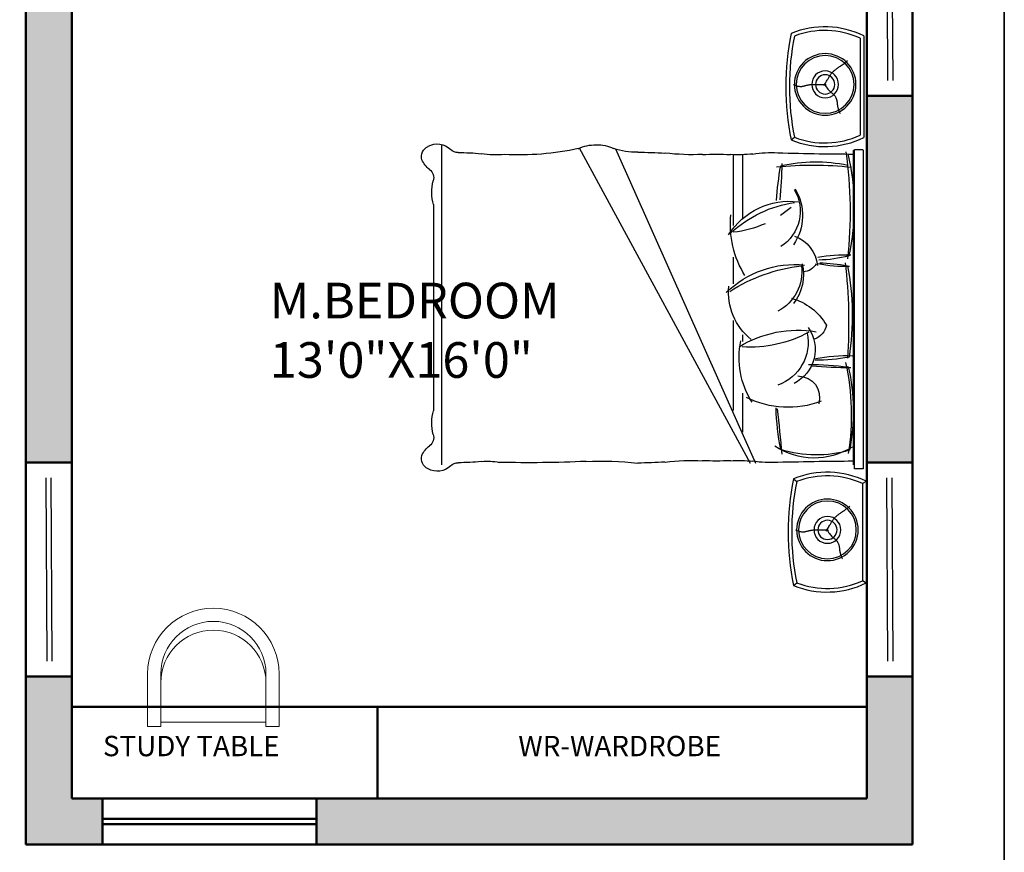
# Model space of a CAD drawing. Units: inches. Extents: x 1986 to 21484, y -1816 to 2016.
# Tile 3 of 85: x 2209 to 2402, y 1113 to 1277. Entities that reach past the tile are written whole.
import ezdxf

# ---------------------------------------------------------------- set-up
doc = ezdxf.new("R2010")
doc.units = ezdxf.units.IN
for name, color, linetype, lineweight in [('A-ANNO-TEXT', 7, 'Continuous', 18), ('A-AREA-IDEN', 3, 'Continuous', 18), ('A-FLOR-FIXT', 8, 'Continuous', 18), ('A-FURN', 8, 'Continuous', 18), ('A-GLAZ', 4, 'Continuous', 25), ('A-WALL', 7, 'Continuous', 50), ('A-WALL-PATT', 8, 'Continuous', 13), ('C-PROP', 7, 'Continuous', 35)]:
    doc.layers.add(name, color=color, linetype=linetype, lineweight=lineweight)
doc.layers.add('TEFRİŞ', color=11, linetype='Continuous')
doc.styles.get("Standard").update_dxf_attribs({"font": 'arial.ttf'})

# ---------------------------------------------------------------- blocks, each defined once
blk = doc.blocks.new('12PSTG07')
at = {"color": 0, "linetype": 'ByBlock'}
for p, q in [((0, 15), (-12, 15)), ((0, 12), (0, 15)), ((-12, 12), (0, 12)), ((-1, -12), (-1, 12)), ((-12, -12), (0, -12)), ((0, -12), (0, -15)), ((0, -15), (-12, -15))]:
    blk.add_line(p, q, dxfattribs=at)
for centre, radius in [((-12, 0), 15), ((-12, 0), 12), ((-10, 0), 12)]:
    blk.add_arc(centre, radius, 90, 270, dxfattribs=at)
blk = doc.blocks.new('BED')
at = {"layer": 'TEFRİŞ'}
for p, q in [((2114.88, 1835.66), (2129.12, 1835.66)), ((2130.81, 1834.34), (2130.81, 1835.55)), ((2130.91, 1835.55), (2175.56, 1835.55)), ((2175.56, 1835.55), (2175.56, 1834.34)), ((2177.29, 1835.98), (2177.61, 1835.47)), ((2177.29, 1835.98), (2191.52, 1835.98)), ((2177.61, 1835.47), (2191.2, 1835.47)), ((2191.2, 1835.47), (2191.52, 1835.98)), ((2115.2, 1835.15), (2128.8, 1835.15)), ((2175.56, 1834.34), (2130.81, 1834.34)), ((2175, 1834.19), (2130.91, 1834.19)), ((2118.49, 1833.2), (2118.34, 1833.38)), ((2118.49, 1833.2), (2118.34, 1833.38)), ((2118.63, 1833.03), (2118.49, 1833.2)), ((2118.63, 1833.03), (2118.49, 1833.2)), ((2118.75, 1832.88), (2118.63, 1833.03)), ((2118.75, 1832.88), (2118.63, 1833.03)), ((2118.86, 1832.74), (2118.75, 1832.88)), ((2118.86, 1832.74), (2118.75, 1832.88)), ((2118.95, 1832.61), (2118.86, 1832.74)), ((2118.95, 1832.61), (2118.86, 1832.74)), ((2119.04, 1832.48), (2118.95, 1832.61)), ((2119.04, 1832.48), (2118.95, 1832.61)), ((2180.9, 1833.52), (2180.75, 1833.7)), ((2180.9, 1833.52), (2180.75, 1833.7)), ((2181.04, 1833.35), (2180.9, 1833.52)), ((2181.04, 1833.35), (2180.9, 1833.52)), ((2181.16, 1833.2), (2181.04, 1833.35)), ((2181.16, 1833.2), (2181.04, 1833.35)), ((2181.26, 1833.06), (2181.16, 1833.2)), ((2181.26, 1833.06), (2181.16, 1833.2)), ((2181.36, 1832.93), (2181.26, 1833.06)), ((2181.36, 1832.93), (2181.26, 1833.06)), ((2181.44, 1832.8), (2181.36, 1832.93)), ((2181.44, 1832.8), (2181.36, 1832.93)), ((2181.52, 1832.69), (2181.44, 1832.8)), ((2181.52, 1832.69), (2181.44, 1832.8)), ((2181.59, 1832.58), (2181.52, 1832.69)), ((2181.59, 1832.58), (2181.52, 1832.69)), ((2181.66, 1832.48), (2181.59, 1832.58)), ((2181.66, 1832.48), (2181.59, 1832.58)), ((2187.83, 1832.49), (2187.92, 1832.53)), ((2187.83, 1832.49), (2187.92, 1832.53)), ((2187.92, 1832.53), (2188.01, 1832.57)), ((2187.92, 1832.53), (2188.01, 1832.57)), ((2188.01, 1832.57), (2188.09, 1832.62)), ((2188.01, 1832.57), (2188.09, 1832.62)), ((2188.09, 1832.62), (2188.15, 1832.67)), ((2188.09, 1832.62), (2188.15, 1832.67)), ((2119.12, 1832.37), (2119.04, 1832.48)), ((2119.12, 1832.37), (2119.04, 1832.48)), ((2119.19, 1832.26), (2119.12, 1832.37)), ((2119.19, 1832.26), (2119.12, 1832.37)), ((2119.26, 1832.16), (2119.19, 1832.26)), ((2119.26, 1832.16), (2119.19, 1832.26)), ((2119.32, 1832.06), (2119.26, 1832.16)), ((2119.32, 1832.06), (2119.26, 1832.16)), ((2119.39, 1831.97), (2119.32, 1832.06)), ((2119.39, 1831.97), (2119.32, 1832.06)), ((2119.45, 1831.89), (2119.39, 1831.97)), ((2119.45, 1831.89), (2119.39, 1831.97)), ((2119.51, 1831.81), (2119.45, 1831.89)), ((2119.51, 1831.81), (2119.45, 1831.89)), ((2119.57, 1831.73), (2119.51, 1831.81)), ((2119.57, 1831.73), (2119.51, 1831.81)), ((2119.63, 1831.65), (2119.57, 1831.73)), ((2119.63, 1831.65), (2119.57, 1831.73)), ((2119.69, 1831.58), (2119.63, 1831.65)), ((2119.69, 1831.58), (2119.63, 1831.65)), ((2119.75, 1831.51), (2119.69, 1831.58)), ((2119.75, 1831.51), (2119.69, 1831.58)), ((2119.81, 1831.44), (2119.75, 1831.51)), ((2119.81, 1831.44), (2119.75, 1831.51)), ((2119.87, 1831.38), (2119.81, 1831.44)), ((2119.87, 1831.38), (2119.81, 1831.44)), ((2119.93, 1831.31), (2119.87, 1831.38)), ((2119.93, 1831.31), (2119.87, 1831.38)), ((2119.99, 1831.25), (2119.93, 1831.31)), ((2119.99, 1831.25), (2119.93, 1831.31)), ((2120.05, 1831.2), (2119.99, 1831.25)), ((2120.05, 1831.2), (2119.99, 1831.25)), ((2120.12, 1831.14), (2120.05, 1831.2)), ((2120.12, 1831.14), (2120.05, 1831.2)), ((2120.18, 1831.09), (2120.12, 1831.14)), ((2120.18, 1831.09), (2120.12, 1831.14)), ((2122.8, 1831.09), (2122.87, 1831.18)), ((2122.8, 1831.09), (2122.87, 1831.18)), ((2122.87, 1831.18), (2122.94, 1831.26)), ((2122.87, 1831.18), (2122.94, 1831.26)), ((2122.94, 1831.26), (2123.01, 1831.33)), ((2122.94, 1831.26), (2123.01, 1831.33)), ((2123.01, 1831.33), (2123.08, 1831.4)), ((2123.01, 1831.33), (2123.08, 1831.4)), ((2123.08, 1831.4), (2123.14, 1831.46)), ((2123.08, 1831.4), (2123.14, 1831.46)), ((2123.14, 1831.46), (2123.21, 1831.52)), ((2123.14, 1831.46), (2123.21, 1831.52)), ((2123.21, 1831.52), (2123.27, 1831.58)), ((2123.21, 1831.52), (2123.27, 1831.58)), ((2123.27, 1831.58), (2123.34, 1831.63)), ((2123.27, 1831.58), (2123.34, 1831.63)), ((2123.34, 1831.63), (2123.41, 1831.67)), ((2123.34, 1831.63), (2123.41, 1831.67)), ((2123.41, 1831.67), (2123.48, 1831.71)), ((2123.41, 1831.67), (2123.48, 1831.71)), ((2123.48, 1831.71), (2123.55, 1831.74)), ((2123.48, 1831.71), (2123.55, 1831.74)), ((2123.55, 1831.74), (2123.62, 1831.77)), ((2123.55, 1831.74), (2123.62, 1831.77)), ((2123.62, 1831.77), (2123.69, 1831.8)), ((2123.62, 1831.77), (2123.69, 1831.8)), ((2123.69, 1831.8), (2123.77, 1831.82)), ((2123.69, 1831.8), (2123.77, 1831.82)), ((2123.77, 1831.82), (2123.84, 1831.84)), ((2123.77, 1831.82), (2123.84, 1831.84)), ((2123.84, 1831.84), (2123.91, 1831.86)), ((2123.84, 1831.84), (2123.91, 1831.86)), ((2123.91, 1831.86), (2123.98, 1831.87)), ((2123.91, 1831.86), (2123.98, 1831.87)), ((2123.98, 1831.87), (2124.06, 1831.89)), ((2123.98, 1831.87), (2124.06, 1831.89)), ((2124.06, 1831.89), (2124.13, 1831.9)), ((2124.06, 1831.89), (2124.13, 1831.9)), ((2124.13, 1831.9), (2124.2, 1831.91)), ((2124.13, 1831.9), (2124.2, 1831.91)), ((2124.2, 1831.91), (2124.27, 1831.91)), ((2124.2, 1831.91), (2124.27, 1831.91)), ((2124.27, 1831.91), (2124.35, 1831.92)), ((2124.27, 1831.91), (2124.35, 1831.92)), ((2124.35, 1831.92), (2124.42, 1831.93)), ((2124.35, 1831.92), (2124.42, 1831.93)), ((2124.42, 1831.93), (2124.49, 1831.94)), ((2124.42, 1831.93), (2124.49, 1831.94)), ((2124.49, 1831.94), (2124.56, 1831.95)), ((2124.49, 1831.94), (2124.56, 1831.95)), ((2124.56, 1831.95), (2124.64, 1831.96)), ((2124.56, 1831.95), (2124.64, 1831.96)), ((2124.64, 1831.96), (2124.71, 1831.98)), ((2124.64, 1831.96), (2124.71, 1831.98)), ((2124.71, 1831.98), (2124.79, 1831.99)), ((2124.71, 1831.98), (2124.79, 1831.99)), ((2124.79, 1831.99), (2124.87, 1832.01)), ((2124.79, 1831.99), (2124.87, 1832.01)), ((2124.87, 1832.01), (2124.96, 1832.03)), ((2124.87, 1832.01), (2124.96, 1832.03)), ((2124.96, 1832.03), (2125.05, 1832.05)), ((2124.96, 1832.03), (2125.05, 1832.05)), ((2125.05, 1832.05), (2125.14, 1832.08)), ((2125.05, 1832.05), (2125.14, 1832.08)), ((2125.14, 1832.08), (2125.23, 1832.11)), ((2125.14, 1832.08), (2125.23, 1832.11)), ((2125.23, 1832.11), (2125.33, 1832.14)), ((2125.23, 1832.11), (2125.33, 1832.14)), ((2125.33, 1832.14), (2125.42, 1832.17)), ((2125.33, 1832.14), (2125.42, 1832.17)), ((2125.42, 1832.17), (2125.52, 1832.21)), ((2125.42, 1832.17), (2125.52, 1832.21)), ((2125.52, 1832.21), (2125.6, 1832.25)), ((2125.52, 1832.21), (2125.6, 1832.25)), ((2125.6, 1832.25), (2125.68, 1832.3)), ((2125.6, 1832.25), (2125.68, 1832.3)), ((2125.68, 1832.3), (2125.75, 1832.35)), ((2125.68, 1832.3), (2125.75, 1832.35)), ((2181.73, 1832.38), (2181.66, 1832.48)), ((2181.73, 1832.38), (2181.66, 1832.48)), ((2181.79, 1832.29), (2181.73, 1832.38)), ((2181.79, 1832.29), (2181.73, 1832.38)), ((2181.85, 1832.21), (2181.79, 1832.29)), ((2181.85, 1832.21), (2181.79, 1832.29)), ((2181.92, 1832.13), (2181.85, 1832.21)), ((2181.92, 1832.13), (2181.85, 1832.21)), ((2181.97, 1832.05), (2181.92, 1832.13)), ((2181.97, 1832.05), (2181.92, 1832.13)), ((2182.03, 1831.97), (2181.97, 1832.05)), ((2182.03, 1831.97), (2181.97, 1832.05)), ((2182.09, 1831.9), (2182.03, 1831.97)), ((2182.09, 1831.9), (2182.03, 1831.97)), ((2182.15, 1831.83), (2182.09, 1831.9)), ((2182.15, 1831.83), (2182.09, 1831.9)), ((2182.21, 1831.76), (2182.15, 1831.83)), ((2182.21, 1831.76), (2182.15, 1831.83)), ((2182.27, 1831.7), (2182.21, 1831.76)), ((2182.27, 1831.7), (2182.21, 1831.76)), ((2182.33, 1831.63), (2182.27, 1831.7)), ((2182.33, 1831.63), (2182.27, 1831.7)), ((2182.4, 1831.57), (2182.33, 1831.63)), ((2182.4, 1831.57), (2182.33, 1831.63)), ((2182.46, 1831.52), (2182.4, 1831.57)), ((2182.46, 1831.52), (2182.4, 1831.57)), ((2182.52, 1831.46), (2182.46, 1831.52)), ((2182.52, 1831.46), (2182.46, 1831.52)), ((2182.59, 1831.41), (2182.52, 1831.46)), ((2182.59, 1831.41), (2182.52, 1831.46)), ((2182.66, 1831.36), (2182.59, 1831.41)), ((2182.66, 1831.36), (2182.59, 1831.41)), ((2182.73, 1831.31), (2182.66, 1831.36)), ((2182.73, 1831.31), (2182.66, 1831.36)), ((2182.8, 1831.26), (2182.73, 1831.31)), ((2182.8, 1831.26), (2182.73, 1831.31)), ((2182.87, 1831.22), (2182.8, 1831.26)), ((2182.87, 1831.22), (2182.8, 1831.26)), ((2182.95, 1831.17), (2182.87, 1831.22)), ((2182.95, 1831.17), (2182.87, 1831.22)), ((2183.03, 1831.12), (2182.95, 1831.17)), ((2183.03, 1831.12), (2182.95, 1831.17)), ((2184.85, 1831.04), (2184.95, 1831.14)), ((2184.85, 1831.04), (2184.95, 1831.14)), ((2184.95, 1831.14), (2185.05, 1831.23)), ((2184.95, 1831.14), (2185.05, 1831.23)), ((2185.05, 1831.23), (2185.13, 1831.33)), ((2185.05, 1831.23), (2185.13, 1831.33)), ((2185.13, 1831.33), (2185.21, 1831.41)), ((2185.13, 1831.33), (2185.21, 1831.41)), ((2185.21, 1831.41), (2185.28, 1831.5)), ((2185.21, 1831.41), (2185.28, 1831.5)), ((2185.28, 1831.5), (2185.35, 1831.58)), ((2185.28, 1831.5), (2185.35, 1831.58)), ((2185.35, 1831.58), (2185.42, 1831.65)), ((2185.35, 1831.58), (2185.42, 1831.65)), ((2185.42, 1831.65), (2185.48, 1831.72)), ((2185.42, 1831.65), (2185.48, 1831.72)), ((2185.48, 1831.72), (2185.55, 1831.78)), ((2185.48, 1831.72), (2185.55, 1831.78)), ((2185.55, 1831.78), (2185.61, 1831.84)), ((2185.55, 1831.78), (2185.61, 1831.84)), ((2185.61, 1831.84), (2185.68, 1831.9)), ((2185.61, 1831.84), (2185.68, 1831.9)), ((2185.68, 1831.9), (2185.75, 1831.95)), ((2185.68, 1831.9), (2185.75, 1831.95)), ((2185.75, 1831.95), (2185.82, 1831.99)), ((2185.75, 1831.95), (2185.82, 1831.99)), ((2185.82, 1831.99), (2185.89, 1832.03)), ((2185.82, 1831.99), (2185.89, 1832.03)), ((2185.89, 1832.03), (2185.96, 1832.06)), ((2185.89, 1832.03), (2185.96, 1832.06)), ((2185.96, 1832.06), (2186.03, 1832.09)), ((2185.96, 1832.06), (2186.03, 1832.09)), ((2186.03, 1832.09), (2186.1, 1832.12)), ((2186.03, 1832.09), (2186.1, 1832.12)), ((2186.1, 1832.12), (2186.17, 1832.14)), ((2186.1, 1832.12), (2186.17, 1832.14)), ((2186.17, 1832.14), (2186.24, 1832.16)), ((2186.17, 1832.14), (2186.24, 1832.16)), ((2186.24, 1832.16), (2186.32, 1832.18)), ((2186.24, 1832.16), (2186.32, 1832.18)), ((2186.32, 1832.18), (2186.39, 1832.19)), ((2186.32, 1832.18), (2186.39, 1832.19)), ((2186.39, 1832.19), (2186.46, 1832.21)), ((2186.39, 1832.19), (2186.46, 1832.21)), ((2186.46, 1832.21), (2186.53, 1832.22)), ((2186.46, 1832.21), (2186.53, 1832.22)), ((2186.53, 1832.22), (2186.61, 1832.23)), ((2186.53, 1832.22), (2186.61, 1832.23)), ((2186.61, 1832.23), (2186.68, 1832.23)), ((2186.61, 1832.23), (2186.68, 1832.23)), ((2186.68, 1832.23), (2186.75, 1832.24)), ((2186.68, 1832.23), (2186.75, 1832.24)), ((2186.75, 1832.24), (2186.82, 1832.25)), ((2186.75, 1832.24), (2186.82, 1832.25)), ((2186.82, 1832.25), (2186.9, 1832.26)), ((2186.82, 1832.25), (2186.9, 1832.26)), ((2186.9, 1832.26), (2186.97, 1832.27)), ((2186.9, 1832.26), (2186.97, 1832.27)), ((2186.97, 1832.27), (2187.04, 1832.28)), ((2186.97, 1832.27), (2187.04, 1832.28)), ((2187.04, 1832.28), (2187.12, 1832.3)), ((2187.04, 1832.28), (2187.12, 1832.3)), ((2187.12, 1832.3), (2187.2, 1832.31)), ((2187.12, 1832.3), (2187.2, 1832.31)), ((2187.2, 1832.31), (2187.28, 1832.33)), ((2187.2, 1832.31), (2187.28, 1832.33)), ((2187.28, 1832.33), (2187.36, 1832.35)), ((2187.28, 1832.33), (2187.36, 1832.35)), ((2187.36, 1832.35), (2187.45, 1832.37)), ((2187.36, 1832.35), (2187.45, 1832.37)), ((2187.45, 1832.37), (2187.54, 1832.4)), ((2187.45, 1832.37), (2187.54, 1832.4)), ((2187.54, 1832.4), (2187.64, 1832.43)), ((2187.54, 1832.4), (2187.64, 1832.43)), ((2187.64, 1832.43), (2187.74, 1832.46)), ((2187.64, 1832.43), (2187.74, 1832.46)), ((2187.74, 1832.46), (2187.83, 1832.49)), ((2187.74, 1832.46), (2187.83, 1832.49)), ((2120.25, 1831.04), (2120.18, 1831.09)), ((2120.25, 1831.04), (2120.18, 1831.09)), ((2120.32, 1830.99), (2120.25, 1831.04)), ((2120.32, 1830.99), (2120.25, 1831.04)), ((2120.39, 1830.94), (2120.32, 1830.99)), ((2120.39, 1830.94), (2120.32, 1830.99)), ((2120.47, 1830.9), (2120.39, 1830.94)), ((2120.47, 1830.9), (2120.39, 1830.94)), ((2120.54, 1830.85), (2120.47, 1830.9)), ((2120.54, 1830.85), (2120.47, 1830.9)), ((2120.62, 1830.8), (2120.54, 1830.85)), ((2120.62, 1830.8), (2120.54, 1830.85)), ((2120.7, 1830.75), (2120.62, 1830.8)), ((2120.7, 1830.75), (2120.62, 1830.8)), ((2120.79, 1830.7), (2120.7, 1830.75)), ((2120.79, 1830.7), (2120.7, 1830.75)), ((2120.88, 1830.65), (2120.79, 1830.7)), ((2120.88, 1830.65), (2120.79, 1830.7)), ((2120.98, 1830.59), (2120.88, 1830.65)), ((2120.98, 1830.59), (2120.88, 1830.65)), ((2121.09, 1830.52), (2120.98, 1830.59)), ((2121.09, 1830.52), (2120.98, 1830.59)), ((2121.21, 1830.45), (2121.09, 1830.52)), ((2121.21, 1830.45), (2121.09, 1830.52)), ((2121.34, 1830.38), (2121.21, 1830.45)), ((2121.34, 1830.38), (2121.21, 1830.45)), ((2121.49, 1830.29), (2121.34, 1830.38)), ((2121.49, 1830.29), (2121.34, 1830.38)), ((2121.66, 1830.21), (2121.49, 1830.29)), ((2121.66, 1830.21), (2121.49, 1830.29)), ((2121.66, 1830.18), (2121.87, 1830.29)), ((2121.66, 1830.18), (2121.87, 1830.29)), ((2121.85, 1830.11), (2121.66, 1830.21)), ((2121.85, 1830.11), (2121.66, 1830.21)), ((2121.74, 1829.99), (2121.73, 1829.83)), ((2121.74, 1829.99), (2121.73, 1829.83)), ((2121.73, 1829.83), (2121.73, 1829.69)), ((2121.73, 1829.83), (2121.73, 1829.69)), ((2121.76, 1830.38), (2121.74, 1830.17)), ((2121.76, 1830.38), (2121.74, 1830.17)), ((2121.74, 1830.17), (2121.74, 1829.99)), ((2121.74, 1830.17), (2121.74, 1829.99)), ((2121.87, 1830.29), (2122.04, 1830.4)), ((2121.87, 1830.29), (2122.04, 1830.4)), ((2122.04, 1830.4), (2122.2, 1830.51)), ((2122.04, 1830.4), (2122.2, 1830.51)), ((2122.2, 1830.51), (2122.33, 1830.61)), ((2122.2, 1830.51), (2122.33, 1830.61)), ((2122.33, 1830.61), (2122.45, 1830.72)), ((2122.33, 1830.61), (2122.45, 1830.72)), ((2122.45, 1830.72), (2122.55, 1830.82)), ((2122.45, 1830.72), (2122.55, 1830.82)), ((2122.55, 1830.82), (2122.64, 1830.91)), ((2122.55, 1830.82), (2122.64, 1830.91)), ((2122.64, 1830.91), (2122.72, 1831.01)), ((2122.64, 1830.91), (2122.72, 1831.01)), ((2122.72, 1831.01), (2122.8, 1831.09)), ((2122.72, 1831.01), (2122.8, 1831.09)), ((2183.11, 1831.07), (2183.03, 1831.12)), ((2183.11, 1831.07), (2183.03, 1831.12)), ((2183.2, 1831.02), (2183.11, 1831.07)), ((2183.2, 1831.02), (2183.11, 1831.07)), ((2183.29, 1830.97), (2183.2, 1831.02)), ((2183.29, 1830.97), (2183.2, 1831.02)), ((2183.39, 1830.91), (2183.29, 1830.97)), ((2183.39, 1830.91), (2183.29, 1830.97)), ((2183.49, 1830.84), (2183.39, 1830.91)), ((2183.49, 1830.84), (2183.39, 1830.91)), ((2183.61, 1830.77), (2183.49, 1830.84)), ((2183.61, 1830.77), (2183.49, 1830.84)), ((2183.75, 1830.7), (2183.61, 1830.77)), ((2183.75, 1830.7), (2183.61, 1830.77)), ((2183.9, 1830.61), (2183.75, 1830.7)), ((2183.9, 1830.61), (2183.75, 1830.7)), ((2184.06, 1830.53), (2183.9, 1830.61)), ((2184.06, 1830.53), (2183.9, 1830.61)), ((2184.25, 1830.43), (2184.06, 1830.53)), ((2184.25, 1830.43), (2184.06, 1830.53)), ((2184.07, 1830.5), (2184.27, 1830.61)), ((2184.07, 1830.5), (2184.27, 1830.61)), ((2184.15, 1830.49), (2184.14, 1830.31)), ((2184.15, 1830.49), (2184.14, 1830.31)), ((2184.14, 1830.31), (2184.14, 1830.15)), ((2184.14, 1830.31), (2184.14, 1830.15)), ((2184.14, 1830.15), (2184.14, 1830.01)), ((2184.14, 1830.15), (2184.14, 1830.01)), ((2184.14, 1830.01), (2184.14, 1829.89)), ((2184.14, 1830.01), (2184.14, 1829.89)), ((2184.14, 1829.89), (2184.14, 1829.77)), ((2184.14, 1829.89), (2184.14, 1829.77)), ((2184.14, 1829.77), (2184.14, 1829.67)), ((2184.14, 1829.77), (2184.14, 1829.67)), ((2184.17, 1830.7), (2184.15, 1830.49)), ((2184.17, 1830.7), (2184.15, 1830.49)), ((2184.27, 1830.61), (2184.45, 1830.72)), ((2184.27, 1830.61), (2184.45, 1830.72)), ((2184.45, 1830.72), (2184.6, 1830.83)), ((2184.45, 1830.72), (2184.6, 1830.83)), ((2184.6, 1830.83), (2184.74, 1830.93)), ((2184.6, 1830.83), (2184.74, 1830.93)), ((2184.74, 1830.93), (2184.85, 1831.04)), ((2184.74, 1830.93), (2184.85, 1831.04)), ((2121.73, 1829.69), (2121.73, 1829.57)), ((2121.73, 1829.69), (2121.73, 1829.57)), ((2121.73, 1829.57), (2121.73, 1829.45)), ((2121.73, 1829.57), (2121.73, 1829.45)), ((2121.73, 1829.45), (2121.74, 1829.35)), ((2121.73, 1829.45), (2121.74, 1829.35)), ((2121.74, 1828.89), (2121.73, 1828.8)), ((2121.74, 1828.89), (2121.73, 1828.8)), ((2121.73, 1828.8), (2121.73, 1828.72)), ((2121.73, 1828.8), (2121.73, 1828.72)), ((2121.73, 1828.72), (2121.73, 1828.64)), ((2121.73, 1828.72), (2121.73, 1828.64)), ((2121.73, 1828.64), (2121.73, 1828.56)), ((2121.73, 1828.64), (2121.73, 1828.56)), ((2121.73, 1828.56), (2121.73, 1828.48)), ((2121.73, 1828.56), (2121.73, 1828.48)), ((2121.73, 1828.48), (2121.73, 1828.4)), ((2121.73, 1828.48), (2121.73, 1828.4)), ((2121.73, 1828.4), (2121.73, 1828.33)), ((2121.73, 1828.4), (2121.73, 1828.33)), ((2121.74, 1829.35), (2121.74, 1829.25)), ((2121.74, 1829.35), (2121.74, 1829.25)), ((2121.74, 1829.25), (2121.74, 1829.16)), ((2121.74, 1829.25), (2121.74, 1829.16)), ((2121.74, 1829.16), (2121.74, 1829.06)), ((2121.74, 1829.16), (2121.74, 1829.06)), ((2121.74, 1829.06), (2121.74, 1828.97)), ((2121.74, 1829.06), (2121.74, 1828.97)), ((2121.74, 1828.97), (2121.74, 1828.89)), ((2121.74, 1828.97), (2121.74, 1828.89)), ((2184.14, 1829.04), (2184.13, 1828.96)), ((2184.14, 1829.04), (2184.13, 1828.96)), ((2184.13, 1828.96), (2184.13, 1828.88)), ((2184.13, 1828.96), (2184.13, 1828.88)), ((2184.13, 1828.88), (2184.13, 1828.8)), ((2184.13, 1828.88), (2184.13, 1828.8)), ((2184.13, 1828.8), (2184.14, 1828.72)), ((2184.13, 1828.8), (2184.14, 1828.72)), ((2184.14, 1829.67), (2184.15, 1829.57)), ((2184.14, 1829.67), (2184.15, 1829.57)), ((2184.15, 1829.38), (2184.14, 1829.29)), ((2184.15, 1829.38), (2184.14, 1829.29)), ((2184.14, 1829.29), (2184.14, 1829.21)), ((2184.14, 1829.29), (2184.14, 1829.21)), ((2184.14, 1829.21), (2184.14, 1829.12)), ((2184.14, 1829.21), (2184.14, 1829.12)), ((2184.14, 1829.12), (2184.14, 1829.04)), ((2184.14, 1829.12), (2184.14, 1829.04)), ((2184.14, 1828.72), (2184.14, 1828.65)), ((2184.14, 1828.72), (2184.14, 1828.65)), ((2184.14, 1828.65), (2184.15, 1828.57)), ((2184.14, 1828.65), (2184.15, 1828.57)), ((2184.15, 1829.57), (2184.15, 1829.48)), ((2184.15, 1829.57), (2184.15, 1829.48)), ((2184.15, 1829.48), (2184.15, 1829.38)), ((2184.15, 1829.48), (2184.15, 1829.38)), ((2184.15, 1828.57), (2184.15, 1828.5)), ((2184.15, 1828.57), (2184.15, 1828.5)), ((2184.15, 1828.5), (2184.16, 1828.42)), ((2184.15, 1828.5), (2184.16, 1828.42)), ((2184.16, 1828.42), (2184.17, 1828.35)), ((2184.16, 1828.42), (2184.17, 1828.35)), ((2121.73, 1828.33), (2121.74, 1828.25)), ((2121.73, 1828.33), (2121.74, 1828.25)), ((2121.74, 1828.25), (2121.75, 1828.18)), ((2121.74, 1828.25), (2121.75, 1828.18)), ((2121.75, 1828.18), (2121.75, 1828.1)), ((2121.75, 1828.18), (2121.75, 1828.1)), ((2121.75, 1828.1), (2121.76, 1828.03)), ((2121.75, 1828.1), (2121.76, 1828.03)), ((2121.76, 1828.03), (2121.78, 1827.95)), ((2121.76, 1828.03), (2121.78, 1827.95)), ((2121.78, 1827.95), (2121.79, 1827.88)), ((2121.78, 1827.95), (2121.79, 1827.88)), ((2121.79, 1827.88), (2121.8, 1827.8)), ((2121.79, 1827.88), (2121.8, 1827.8)), ((2121.8, 1827.8), (2121.82, 1827.72)), ((2121.8, 1827.8), (2121.82, 1827.72)), ((2121.82, 1827.72), (2121.84, 1827.65)), ((2121.82, 1827.72), (2121.84, 1827.65)), ((2121.84, 1827.65), (2121.85, 1827.57)), ((2121.84, 1827.65), (2121.85, 1827.57)), ((2121.85, 1827.57), (2121.87, 1827.49)), ((2121.85, 1827.57), (2121.87, 1827.49)), ((2121.87, 1827.49), (2121.89, 1827.41)), ((2121.87, 1827.49), (2121.89, 1827.41)), ((2121.89, 1827.41), (2121.91, 1827.33)), ((2121.89, 1827.41), (2121.91, 1827.33)), ((2121.91, 1827.33), (2121.93, 1827.26)), ((2121.91, 1827.33), (2121.93, 1827.26)), ((2121.93, 1827.26), (2121.95, 1827.18)), ((2121.93, 1827.26), (2121.95, 1827.18)), ((2121.95, 1827.18), (2121.97, 1827.09)), ((2121.95, 1827.18), (2121.97, 1827.09)), ((2121.97, 1827.09), (2121.99, 1827.01)), ((2121.97, 1827.09), (2121.99, 1827.01)), ((2121.99, 1827.01), (2122, 1826.93)), ((2121.99, 1827.01), (2122, 1826.93)), ((2184.17, 1828.35), (2184.18, 1828.27)), ((2184.17, 1828.35), (2184.18, 1828.27)), ((2184.18, 1828.27), (2184.19, 1828.2)), ((2184.18, 1828.27), (2184.19, 1828.2)), ((2184.19, 1828.2), (2184.21, 1828.12)), ((2184.19, 1828.2), (2184.21, 1828.12)), ((2184.21, 1828.12), (2184.22, 1828.04)), ((2184.21, 1828.12), (2184.22, 1828.04)), ((2184.22, 1828.04), (2184.24, 1827.97)), ((2184.22, 1828.04), (2184.24, 1827.97)), ((2184.24, 1827.97), (2184.26, 1827.89)), ((2184.24, 1827.97), (2184.26, 1827.89)), ((2184.26, 1827.89), (2184.28, 1827.81)), ((2184.26, 1827.89), (2184.28, 1827.81)), ((2184.28, 1827.81), (2184.3, 1827.73)), ((2184.28, 1827.81), (2184.3, 1827.73)), ((2184.3, 1827.73), (2184.32, 1827.65)), ((2184.3, 1827.73), (2184.32, 1827.65)), ((2184.32, 1827.65), (2184.34, 1827.58)), ((2184.32, 1827.65), (2184.34, 1827.58)), ((2184.34, 1827.58), (2184.36, 1827.5)), ((2184.34, 1827.58), (2184.36, 1827.5)), ((2184.36, 1827.5), (2184.38, 1827.41)), ((2184.36, 1827.5), (2184.38, 1827.41)), ((2184.38, 1827.41), (2184.4, 1827.33)), ((2184.38, 1827.41), (2184.4, 1827.33)), ((2184.4, 1827.33), (2184.41, 1827.25)), ((2184.4, 1827.33), (2184.41, 1827.25)), ((2184.41, 1827.06), (2184.4, 1826.96)), ((2184.41, 1827.06), (2184.4, 1826.96)), ((2184.41, 1827.25), (2184.41, 1827.16)), ((2184.41, 1827.25), (2184.41, 1827.16)), ((2184.41, 1827.16), (2184.41, 1827.06)), ((2184.41, 1827.16), (2184.41, 1827.06)), ((2121.78, 1825.93), (2121.74, 1825.8)), ((2121.78, 1825.93), (2121.74, 1825.8)), ((2121.83, 1826.06), (2121.78, 1825.93)), ((2121.83, 1826.06), (2121.78, 1825.93)), ((2121.87, 1826.19), (2121.83, 1826.06)), ((2121.87, 1826.19), (2121.83, 1826.06)), ((2121.91, 1826.31), (2121.87, 1826.19)), ((2121.91, 1826.31), (2121.87, 1826.19)), ((2121.95, 1826.42), (2121.91, 1826.31)), ((2121.95, 1826.42), (2121.91, 1826.31)), ((2121.97, 1826.54), (2121.95, 1826.42)), ((2121.97, 1826.54), (2121.95, 1826.42)), ((2121.99, 1826.64), (2121.97, 1826.54)), ((2121.99, 1826.64), (2121.97, 1826.54)), ((2122, 1826.74), (2121.99, 1826.64)), ((2122, 1826.74), (2121.99, 1826.64)), ((2122, 1826.93), (2122.01, 1826.84)), ((2122, 1826.93), (2122.01, 1826.84)), ((2122.01, 1826.84), (2122, 1826.74)), ((2122.01, 1826.84), (2122, 1826.74)), ((2129.46, 1825.49), (2129.09, 1825.93)), ((2176.94, 1825.81), (2177.31, 1826.25)), ((2184.19, 1826.25), (2184.14, 1826.12)), ((2184.19, 1826.25), (2184.14, 1826.12)), ((2184.23, 1826.38), (2184.19, 1826.25)), ((2184.23, 1826.38), (2184.19, 1826.25)), ((2184.28, 1826.51), (2184.23, 1826.38)), ((2184.28, 1826.51), (2184.23, 1826.38)), ((2184.32, 1826.63), (2184.28, 1826.51)), ((2184.32, 1826.63), (2184.28, 1826.51)), ((2184.35, 1826.74), (2184.32, 1826.63)), ((2184.35, 1826.74), (2184.32, 1826.63)), ((2184.38, 1826.86), (2184.35, 1826.74)), ((2184.38, 1826.86), (2184.35, 1826.74)), ((2184.4, 1826.96), (2184.38, 1826.86)), ((2184.4, 1826.96), (2184.38, 1826.86)), ((2191.87, 1825.81), (2191.5, 1826.25)), ((2174.77, 1820.53), (2130.76, 1800.91)), ((2174.77, 1819.77), (2130.6, 1795.83)), ((2140.43, 1818.69), (2131.53, 1818.69)), ((2141.43, 1817.4), (2131.53, 1817.4)), ((2149.62, 1817.4), (2145.88, 1817.4)), ((2167.36, 1817.4), (2154.77, 1817.4)), ((2157.71, 1818.69), (2156.77, 1818.69)), ((2170.41, 1818.69), (2164.92, 1818.69)), ((2175, 1776.57), (2130.11, 1776.57)), ((2138.52, 1775.41), (2167.39, 1775.41))]:
    blk.add_line(p, q, dxfattribs=at)
for centre, radius, start, end in [((2126, 1830.19), 12.39, 153.8162, 202.314), ((2118, 1830.19), 12.39, 337.686, 26.1838), ((2188.4, 1830.51), 12.39, 153.8162, 202.314), ((2188.4, 1830.51), 11.88, 155.3335, 201.0157), ((2180.41, 1830.51), 11.88, 338.9843, 24.6665), ((2180.41, 1830.51), 12.39, 337.686, 26.1838), ((2126, 1830.19), 11.88, 155.3335, 201.0157), ((2118, 1830.19), 11.88, 338.9843, 24.6665), ((2122, 1861.35), 36.12, 258.6773, 281.3227), ((2184.41, 1861.67), 36.63, 258.2443, 281.7557), ((2184.41, 1861.67), 36.12, 258.6773, 281.3227), ((2122, 1861.35), 36.63, 258.2443, 281.7557)]:
    blk.add_arc(centre, radius, start, end, dxfattribs=at)
at = {"layer": 'TEFRİŞ', "extrusion": (0, 0, -1)}
for centre, major_axis, ratio, start_param, end_param in [((2121.68, 1830.24), (-3.05, -3.05), 1, 3.926991, 10.210176), ((2121.68, 1830.24), (2.86, -2.86), 1, 5.497787, 11.780972), ((2121.68, 1830.24), (2.86, -2.86), 1, 5.497787, 11.780972), ((2139.43, 1773.84), (-42.35, 42.35), 1, 0.646251, 0.896949), ((2206.14, 1830.73), (-52.86, -52.86), 1, 0.767743, 0.83177), ((2138.85, 1803.05), (-22.1, 22.1), 1, 0.544604, 1.006234), ((2181.61, 1828.44), (-34.39, 34.39), 1, -0.888486, -0.672463), ((2154.12, 1796.61), (-26.46, 26.46), 1, 0.596409, 0.940188), ((2183.72, 1833.22), (-17, 17), 1, -0.967105, -0.749712), ((2168.35, 1789.27), (-1.33, 44.62), 0.875277, -0.163954, 0.163954), ((2167.6, 1797.72), (-0.51, 36.47), 0.865194, -0.185965, 0.185965), ((2164.15, 1828.7), (-6.99, 6.99), 1, 1.789136, 2.946702), ((2099.77, 1830.73), (-52.86, 52.86), 1, 2.311571, 2.373849), ((2184.09, 1830.56), (-3.05, -3.05), 1, 3.926991, 10.210176), ((2184.09, 1830.56), (2.86, -2.86), 1, 5.497787, 11.780972), ((2184.09, 1830.56), (2.86, -2.86), 1, 5.497787, 11.780972), ((2154.7, 1828.89), (-15.68, 15.68), 1, -1.00675, -0.580436), ((2164.51, 1832.79), (-13.41, 13.41), 1, -0.974476, -0.730892), ((2127.6, 1828.81), (-13.23, 13.23), 1, 2.100388, 2.328052), ((2155, 1761.9), (-50.65, -50.65), 1, 2.239512, 2.426533), ((2172.01, 1828.66), (-17.93, 17.93), 1, -0.753394, -0.598744), ((2128.44, 1832.96), (-13.26, -13.26), 1, 3.889049, 4.127298), ((2134, 1828.8), (-18.62, 18.62), 1, 2.173461, 2.355043), ((2199.2, 1828.45), (-27.06, -27.06), 1, 0.770625, 0.917228), ((2087.32, 1833.96), (-52.37, 52.37), 1, 2.358049, 2.431787), ((2156.76, 1828.98), (-11.9, -11.9), 1, 3.646453, 4.226155), ((2121.68, 1830.24), (1.33, -1.33), 1, 5.497787, 11.780972), ((2121.68, 1830.24), (1.33, -1.33), 1, 5.497787, 11.780972), ((2121.68, 1830.24), (0.952, -0.952), 1, 5.497787, 11.780972), ((2121.68, 1830.24), (0.952, -0.952), 1, 5.497787, 11.780972), ((2184.09, 1830.56), (1.33, -1.33), 1, 5.497787, 11.780972), ((2184.09, 1830.56), (1.33, -1.33), 1, 5.497787, 11.780972), ((2184.09, 1830.56), (0.952, -0.952), 1, 5.497787, 11.780972), ((2184.09, 1830.56), (0.952, -0.952), 1, 5.497787, 11.780972), ((2159.55, 1823.33), (-5.81, 5.81), 1, -0.516587, 0.256776), ((2154.84, 1827.75), (-1.93, 1.93), 1, 0.997904, 1.977819), ((2166.67, 1824.96), (-2.93, 3.91), 0.760601, -0.723751, 0.723751), ((2675.38, 1815.09), (-384.79, -384.79), 1, 0.80103, 0.811711), ((2147.44, 1824.41), (-3.36, -3.36), 1, 1.11934, 2.270556), ((2145.66, 1827.01), (-1.62, 1.62), 1, 1.310976, 2.284591), ((2172, 1826.44), (-11.23, 11.23), 1, -1.332486, -0.624868), ((2158.82, 1823.55), (-3.74, -3.74), 1, 1.730792, 3.47045), ((2153.88, 1825.05), (-9.22, 9.22), 1, 1.994956, 2.818753), ((1630.53, 1815.09), (-384.79, 384.79), 1, 2.329881, 2.340562), ((2140.05, 1819.86), (-5.1, 5.1), 1, 0.238357, 1.390139), ((2139.42, 1820.79), (-4.21, -4.21), 1, 1.82161, 3.349145), ((2160.6, 1825.98), (-9.68, -9.68), 1, 0.009196, 0.886853), ((2148.35, 1820.65), (-4.63, -4.63), 1, 2.117602, 3.020837), ((2147.86, 1820.64), (-4.48, 4.48), 1, 0.665914, 1.867503), ((2141.71, 1819.83), (-11.86, 11.86), 1, 1.850844, 2.42862), ((2157.83, 1821.53), (-4.47, 4.47), 1, 0.576679, 2.021689), ((2148.15, 1825.25), (-7.14, -7.14), 1, 6.061986, 7.190757), ((2154.93, 1828.48), (-11.96, 11.96), 1, -1.530302, -0.934407), ((2170.68, 1829.67), (-16.79, 16.79), 1, -1.354718, -0.902276), ((2127.37, 1815.76), (-10.68, 10.68), 1, 1.657204, 1.779381), ((2146.08, 1822.57), (-10.5, 10.5), 1, -0.951783, -0.716225), ((2132.43, 1774.09), (-35.41, -35.41), 1, 2.362911, 2.464592), ((2140.17, 1862.96), (-27.99, 27.99), 1, 3.983025, 4.107469), ((2165.73, 1860.69), (-26.41, -26.41), 1, 5.306413, 5.463767), ((2199.62, 1529.47), (-209.2, 209.2), 1, 0.675361, 0.697001), ((2159.82, 1822.57), (-10.5, -10.5), 1, 3.857817, 4.093375), ((2127.37, 1815.76), (-10.68, 10.68), 1, 1.94252, 2.248924), ((2111.06, 1818.12), (-14.48, 14.48), 1, 2.258605, 2.412359), ((2194.85, 1818.12), (-14.48, 14.48), 1, -0.841563, -0.687809), ((2141.33, 1830.48), (-9.55, -9.55), 1, 4.941413, 5.601673), ((2150.79, 1825.18), (-6, 6), 1, 3.032122, 4.026148), ((2159.02, 1834.9), (-3.04, 16.53), 0.830169, 2.822117, 3.461068), ((2169.92, 1815.01), (-27.2, -27.2), 1, 0.734393, 0.836404), ((2135.98, 1815.01), (-27.2, -27.2), 1, 3.875985, 3.977996), ((2098.24, 1811.68), (-23.54, -23.54), 1, 3.885834, 4.043401), ((2207.66, 1811.68), (-23.54, -23.54), 1, 0.668988, 0.826555), ((2189.03, 1803.74), (-40.91, -40.91), 1, 0.789771, 0.855756), ((2116.87, 1803.74), (-40.91, 40.91), 1, 2.285836, 2.351822), ((2122.14, 1803.63), (-6.39, -6.39), 1, 3.886359, 4.265474), ((2222.76, 1798.77), (-34.16, -34.16), 1, 0.743488, 0.893627), ((2135.02, 1798.41), (-3.45, 3.45), 1, -0.831635, -0.314979), ((2135.48, 1798), (-3.77, -3.77), 1, 0.329385, 0.820948), ((2148.06, 1790.38), (-0.75, 67.37), 0.394952, 1.480524, 1.661068), ((2127.76, 1790.23), (-1, 12.37), 0.296708, 1.141067, 2.000525), ((2118.49, 1784.2), (-9.24, -9.24), 1, 3.839645, 4.088086), ((2182.27, 1782.99), (-5.52, -5.52), 1, 0.671703, 0.993321), ((2162.12, 1778.86), (-21.85, 21.85), 1, -0.78611, -0.680117), ((2143.78, 1778.86), (-21.85, 21.85), 1, 2.250913, 2.356906), ((2129.83, 1778.8), (-0.986, 0.986), 1, 2.330985, 3.163296), ((2176.08, 1778.8), (-0.986, 0.986), 1, 4.690686, 5.522997), ((2132.72, 1775.92), (-1.91, -1.91), 1, 0.284117, 1.557111), ((2173.18, 1775.92), (-1.91, -1.91), 1, 3.155278, 4.428271), ((2131.79, 1775.28), (-1.11, 1.11), 1, 3.629269, 5.067473), ((2130.83, 1777), (-2.49, -2.49), 1, 4.590984, 5.084038), ((2134.73, 1774.06), (-0.964, -0.964), 1, 1.381176, 2.701227), ((2136.75, 1781.14), (-4.24, 4.24), 1, 3.62713, 4.188813), ((2169.16, 1781.14), (-4.24, 4.24), 1, 3.665169, 4.226852), ((2171.17, 1774.06), (-0.964, -0.964), 1, 2.011162, 3.331212), ((2175.07, 1777), (-2.49, 2.49), 1, 4.34074, 4.833793), ((2174.12, 1775.28), (-1.11, 1.11), 1, 2.786508, 4.224712)]:
    blk.add_ellipse(centre, major_axis=major_axis, ratio=ratio, start_param=start_param, end_param=end_param, dxfattribs=at)
blk = doc.blocks.new('WIN-36')
for p, q in [((0, 36), (0, 0)), ((0, 36), (0, 0)), ((1, 36), (1, 0))]:
    blk.add_line(p, q)

msp = doc.modelspace()

# ---------------------------------------------------------------- hatches: boundary and pattern name
at = {"layer": 'A-WALL-PATT'}
h = msp.add_hatch(color=256, dxfattribs=at)
h.dxf.hatch_style = 1
h.paths.add_polyline_path([(2087.31, 1843.75), (2135.31, 1843.75), (2135.31, 1852.75), (2078.31, 1852.75), (2078.31, 1753.75), (2087.31, 1753.75)])
h.paths.add_polyline_path([(2231.31, 1852.75), (2177.31, 1852.75), (2177.31, 1843.75), (2225.31, 1843.75), (2225.31, 1627.75), (2231.31, 1627.75), (2231.31, 1633.35), (2231.31, 1676.45), (2231.31, 1678.13)])
h.paths.add_polyline_path([(2384.31, 1852.75), (2261.31, 1852.75), (2261.31, 1843.75), (2375.31, 1843.75), (2375.31, 1795.75), (2279.31, 1795.75), (2279.31, 1813.75), (2273.31, 1813.75), (2273.31, 1789.75), (2375.31, 1789.75), (2375.31, 1741.75), (2384.31, 1741.75)])
h.paths.add_polyline_path([(2384.31, 1705.75), (2375.31, 1705.75), (2375.31, 1600.75), (2384.31, 1600.75)])
h.paths.add_polyline_path([(2384.31, 1564.75), (2375.31, 1564.75), (2375.31, 1537.75), (2293.31, 1537.75), (2293.31, 1531.75), (2375.31, 1531.75), (2384.31, 1531.75)])
h.paths.add_polyline_path([(2087.31, 1711.75), (2078.31, 1711.75), (2078.31, 1669.75), (2087.31, 1669.75), (2087.31, 1681.75), (2177.31, 1681.75), (2177.31, 1663.75), (2183.31, 1663.75), (2183.31, 1681.75), (2189.31, 1681.75), (2189.31, 1687.75), (2087.31, 1687.75)])
h.paths.add_polyline_path([(2087.31, 1627.75), (2183.31, 1627.75), (2183.31, 1633.75), (2153.31, 1633.75), (2087.31, 1633.75), (2087.31, 1645.75), (2078.31, 1645.75), (2078.31, 1441.75), (2087.31, 1441.75)])
h.paths.add_polyline_path([(2087.31, 1399.75), (2078.31, 1399.75), (2078.31, 1276.75), (2087.31, 1276.75)])
h.paths.add_polyline_path([(2151.81, 1387.75), (2135.31, 1387.75), (2135.31, 1378.75), (2151.81, 1378.75)])
h.paths.add_polyline_path([(2219.31, 1387.75), (2193.81, 1387.75), (2193.81, 1378.75), (2210.31, 1378.75), (2210.31, 1189.75), (2219.31, 1189.75)])
h.paths.add_polyline_path([(2384.31, 1387.75), (2375.31, 1387.75), (2255.31, 1387.75), (2255.31, 1381.75), (2375.31, 1381.75), (2375.31, 1363.75), (2384.31, 1363.75)])
h.paths.add_polyline_path([(2384.31, 1339.75), (2375.31, 1339.75), (2375.31, 1321.75), (2279.31, 1321.75), (2279.31, 1351.75), (2273.31, 1351.75), (2273.31, 1315.75), (2375.31, 1315.75), (2375.31, 1303.75), (2384.31, 1303.75)])
h.paths.add_polyline_path([(2225.31, 1123.75), (2219.31, 1123.75), (2219.31, 1147.75), (2210.31, 1147.75), (2210.31, 1114.75), (2225.31, 1114.75)])
h.paths.add_polyline_path([(2384.31, 1147.75), (2375.31, 1147.75), (2375.31, 1123.75), (2267.31, 1123.75), (2267.31, 1114.75), (2384.31, 1114.75)])
h.paths.add_polyline_path([(2384.31, 1261.75), (2375.31, 1261.75), (2375.31, 1189.75), (2384.31, 1189.75)])
h.paths.add_polyline_path([(2384.31, 1441.75), (2375.31, 1441.75), (2375.31, 1423.75), (2384.31, 1423.75)])
h.paths.add_polyline_path([(2384.31, 1495.75), (2375.31, 1495.75), (2375.31, 1477.75), (2384.31, 1477.75)])

# ---------------------------------------------------------------- linework, layer by layer
at = {"layer": 'A-WALL'}
for p, q in [((2384.31, 1900.75), (2384.31, 1114.75)), ((2219.31, 1123.75), (2219.31, 1387.75)), ((2210.31, 1114.75), (2210.31, 1378.75)), ((2375.31, 1315.75), (2375.31, 1123.75)), ((2375.31, 1261.75), (2384.31, 1261.75)), ((2210.31, 1189.75), (2219.31, 1189.75)), ((2375.31, 1189.75), (2384.31, 1189.75)), ((2210.31, 1147.75), (2219.31, 1147.75)), ((2375.31, 1147.75), (2384.31, 1147.75)), ((2219.31, 1141.75), (2375.31, 1141.75)), ((2279.31, 1123.75), (2279.31, 1141.75)), ((2219.31, 1123.75), (2375.31, 1123.75)), ((2225.31, 1114.75), (2225.31, 1123.75)), ((2267.31, 1114.75), (2267.31, 1123.75)), ((2225.31, 1119.75), (2267.31, 1119.75)), ((2225.31, 1118.75), (2267.31, 1118.75)), ((2384.31, 1114.75), (2210.31, 1114.75))]:
    msp.add_line(p, q, dxfattribs=at)
at = {"layer": 'C-PROP'}
msp.add_lwpolyline([(2042.31, 1900.75), (2402.31, 1900.75), (2402.31, 1066.75), (2042.31, 1066.75)], close=True, dxfattribs=at)

# ---------------------------------------------------------------- block references
at = {"layer": 'A-FLOR-FIXT', "xscale": 0.8597921787217941, "yscale": 0.8597921787217941, "zscale": 0.8597921787217941, "rotation": 270}
msp.add_blockref('12PSTG07', (2247.09, 1137.91), dxfattribs=at)
at = {"layer": 'A-FURN', "xscale": 1.401381342801572, "yscale": 1.401381342801572, "zscale": 1.401381342801572, "rotation": 270}
msp.add_blockref('BED', (-197.71, 4237.25), dxfattribs=at)
at = {"layer": 'A-GLAZ', "rotation": 0.302793432207276}
for p in [(2379.41, 1264.75), (2214.41, 1150.75), (2379.41, 1150.75)]:
    msp.add_blockref('WIN-36', p, dxfattribs=at)

# ---------------------------------------------------------------- texts
at = {"layer": 'A-ANNO-TEXT', "char_height": 4, "attachment_point": 1}
for s, insert in [('{\\fTimes New Roman|b0|i0|c0|p18;STUDY TABLE}', (2225.42, 1136.07)), ('{\\fTimes New Roman|b0|i0|c0|p18;WR-WARDROBE}', (2306.93, 1136.07))]:
    msp.add_mtext_dynamic_manual_height_columns(s, width=105.6127, gutter_width=12.5, heights=[0], dxfattribs=dict(at, insert=insert))
at = {"layer": 'A-AREA-IDEN', "insert": (2258.17, 1225.03), "char_height": 7, "attachment_point": 1}
msp.add_mtext_dynamic_manual_height_columns('{\\fTimes New Roman|b0|i0|c0|p18;M.BEDROOM \\P13\'0"X16\'0"}', width=105.6127, gutter_width=12.5, heights=[0], dxfattribs=at)

doc.saveas('drawing.dxf')
